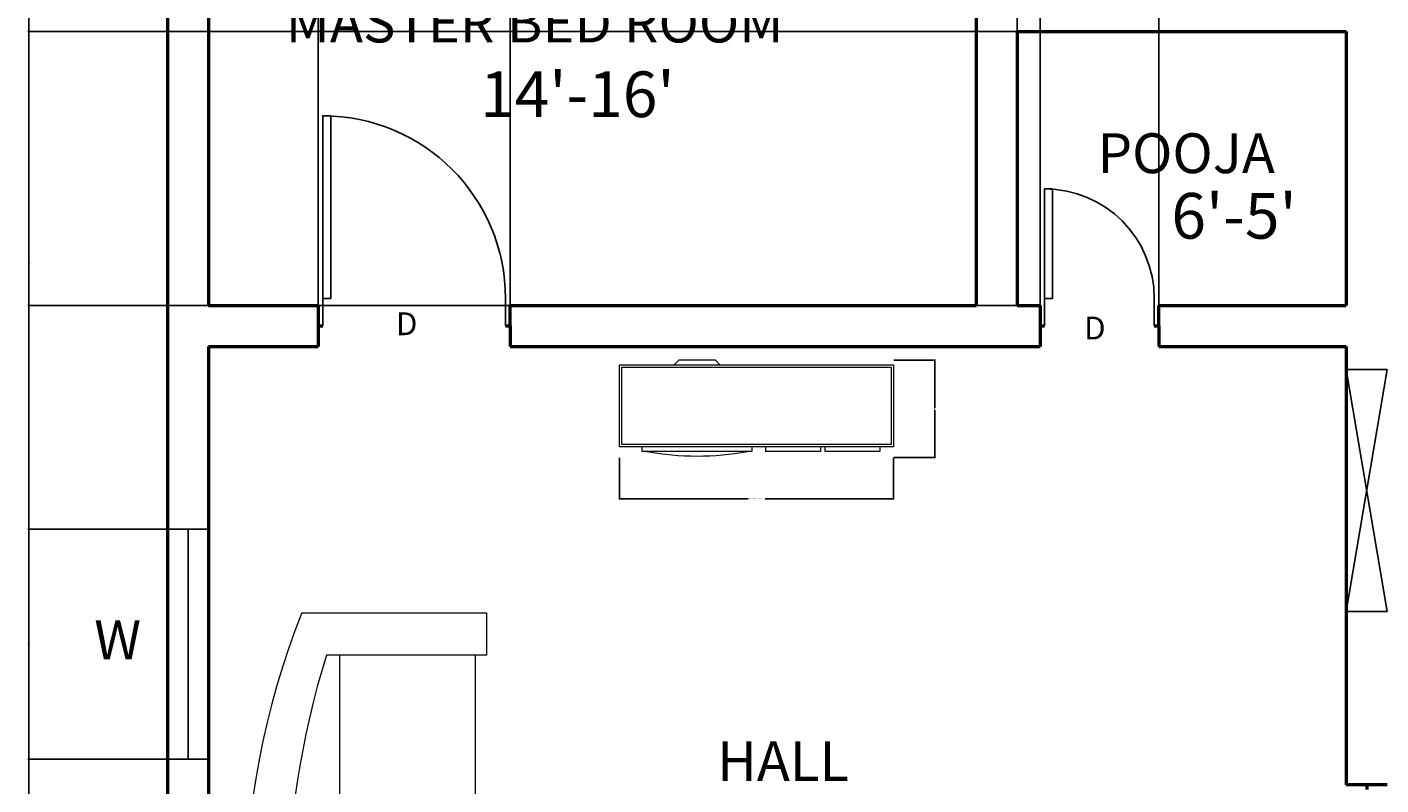
# Model space of a CAD drawing. Units: inches. Extents: x 2164 to 3752, y 2015 to 2629.
# Tile 2 of 8: x 2164 to 2461, y 2223 to 2389. Entities that reach past the tile are written whole.
import ezdxf
from ezdxf.enums import TextEntityAlignment as Align

# ---------------------------------------------------------------- set-up
doc = ezdxf.new("R2010")
doc.units = ezdxf.units.IN
for name, color, linetype, lineweight in [('A-ANNO-DIMS', 2, 'Continuous', 18), ('A-ANNO-TEXT', 7, 'Continuous', 25), ('A-AREA-IDEN', 3, 'Continuous', 25), ('A-DOOR', 3, 'Continuous', 25), ('A-FURN', 8, 'Continuous', 18), ('A-GLAZ', 4, 'Continuous', 25), ('A-WALL', 7, 'Continuous', 50)]:
    doc.layers.add(name, color=color, linetype=linetype, lineweight=lineweight)
doc.styles.get("Standard").update_dxf_attribs({"font": 'arial.ttf'})
doc.dimstyles.get("Standard").update_dxf_attribs({"dimtxt": 0.18, "dimasz": 0.18, "dimexe": 0.18, "dimexo": 0.0625, "dimgap": 0.09, "dimtad": 0, "dimtih": 1, "dimtoh": 1, "dimdec": 4, "dimzin": 0, "dimdsep": 46, "dimtxsty": 'Standard', "dimcen": 0.09, "dimadec": 0, "dimazin": 0, "dimtfac": 1, "dimtdec": 4, "dimtofl": 0, "dimtmove": 0, "dimatfit": 3, "dimfxl": 1, "dimtolj": 1, "dimtzin": 0, "dimarcsym": 0})

# ---------------------------------------------------------------- blocks, each defined once
blk = doc.blocks.new('Sofa - Roundback 7 ft.')
for p, q in [((-12.00002, -32.4421), (-12.00003, -6.5971)), ((11.99997, -32.4421), (11.99998, -6.5971)), ((-36.000027, -34), (-36.000027, -11.4696)), ((35.99998, -34), (35.99998, -11.4696)), ((-35.999844, -13.3819), (35.9998, -13.3819)), ((-36.000027, -32.4421), (35.99998, -32.4421))]:
    blk.add_line(p, q)
for points in [[(-36.000027, -34), (-42.000027, -34), (-42.000027, -8)], [(41.99998, -8), (41.99998, -34), (35.99998, -34)]]:
    blk.add_lwpolyline(points)
for centre, radius, start, end in [((0, -114.25), 114.25, 68.43141, 111.5686), ((-0.00001, -127.1968), 121.1968, 72.72033, 107.2797)]:
    blk.add_arc(centre, radius, start, end)
blk = doc.blocks.new('*U2')
for p, q in [((0, 0), (0, -6)), ((24, 0), (24, -6))]:
    blk.add_line(p, q)
blk.add_lwpolyline([(0, 0), (0, 24), (1.75, 24), (1.75, 0)], close=True)
blk.add_arc((0, 0), 24, 0, 90)
blk = doc.blocks.new('Entertainment Center')
for p, q in [((-4, 0), (-5, -1)), ((4, 0), (-4, 0)), ((5, -1), (4, 0)), ((-17, -19), (-17, -1)), ((-17, -1), (43, -1)), ((-16.5, -18.5), (-16.5, -1.5)), ((-16.5, -1.5), (42.5, -1.5)), ((42.5, -1.5), (42.5, -18.5)), ((43, -1), (43, -19)), ((43, -19), (-17, -19)), ((42.5, -18.5), (-16.5, -18.5)), ((-12, -20), (-12, -19)), ((12, -20), (-12, -20)), ((12, -19), (12, -20)), ((15, -20), (15, -19)), ((27, -20), (15, -20)), ((27, -19), (27, -20)), ((28, -20), (28, -19)), ((40, -20), (28, -20)), ((40, -19), (40, -20))]:
    blk.add_line(p, q)
blk.add_arc((0, 40), 61, 259.6111, 280.3889)
blk = doc.blocks.new('*U7')
for p, q in [((0, 0), (0, -6)), ((40, 0), (40, -6))]:
    blk.add_line(p, q)
blk.add_lwpolyline([(0, 0), (0, 40), (1.75, 40), (1.75, 0)], close=True)
blk.add_arc((0, 0), 40, 0, 90)
blk = doc.blocks.new('VENT-OPENING')
for p, q in [((9, 53), (0, 53)), ((9, 53), (0, 0)), ((9, 0), (0, 53)), ((9, 0), (0, 0))]:
    blk.add_line(p, q)
blk = doc.blocks.new('*D43')
at = {"layer": 'A-ANNO-DIMS', "color": 0, "lineweight": -2, "transparency": 16777216}
for p, q in [((2294.06, 2294.33), (2294.06, 2285.21)), ((2354.06, 2294.33), (2354.06, 2285.21)), ((2294.24, 2285.39), (2322.19, 2285.39)), ((2353.88, 2285.39), (2325.93, 2285.39))]:
    blk.add_line(p, q, dxfattribs=at)
at = {"layer": 'A-ANNO-DIMS', "color": 0, "transparency": 16777216}
for points in [[(2294.24, 2285.42), (2294.24, 2285.36), (2294.06, 2285.39)], [(2353.88, 2285.42), (2353.88, 2285.36), (2354.06, 2285.39)]]:
    blk.add_solid(points, dxfattribs=at)
at = {"layer": 'Defpoints', "color": 0, "transparency": 16777216}
for p in [(2294.06, 2294.39), (2354.06, 2294.39), (2354.06, 2285.39)]:
    blk.add_point(p, dxfattribs=at)
at = {"layer": 'A-ANNO-DIMS', "color": 0, "transparency": 16777216, "insert": (2324.06, 2285.39), "char_height": 0.18, "attachment_point": 5}
blk.add_mtext('\\A1;ENTERTAINMENT CENTER 60', dxfattribs=at)
blk = doc.blocks.new('*D44')
at = {"layer": 'A-ANNO-DIMS', "color": 0, "lineweight": -2, "transparency": 16777216}
for p, q in [((2354.12, 2315.73), (2363.24, 2315.73)), ((2363.06, 2315.55), (2363.06, 2305.24)), ((2363.06, 2294.57), (2363.06, 2304.88)), ((2354.12, 2294.39), (2363.24, 2294.39))]:
    blk.add_line(p, q, dxfattribs=at)
at = {"layer": 'A-ANNO-DIMS', "color": 0, "transparency": 16777216}
for points in [[(2363.03, 2315.55), (2363.09, 2315.55), (2363.06, 2315.73)], [(2363.03, 2294.57), (2363.09, 2294.57), (2363.06, 2294.39)]]:
    blk.add_solid(points, dxfattribs=at)
at = {"layer": 'Defpoints', "color": 0, "transparency": 16777216}
for p in [(2354.06, 2315.73), (2363.06, 2315.73), (2354.06, 2294.39)]:
    blk.add_point(p, dxfattribs=at)
at = {"layer": 'A-ANNO-DIMS', "color": 0, "transparency": 16777216, "insert": (2363.06, 2305.06), "char_height": 0.18, "attachment_point": 5}
blk.add_mtext('\\A1;21', dxfattribs=at)
blk = doc.blocks.new('*D70')
at = {"layer": 'A-ANNO-DIMS', "color": 0, "lineweight": -2, "transparency": 16777216}
for p, q in [((2195.05, 2228.35), (2164.58, 2228.35)), ((2164.76, 2228.17), (2164.76, 2202)), ((2164.76, 2175.46), (2164.76, 2201.63)), ((2195.05, 2175.28), (2164.58, 2175.28))]:
    blk.add_line(p, q, dxfattribs=at)
at = {"layer": 'A-ANNO-DIMS', "color": 0, "transparency": 16777216}
for points in [[(2164.73, 2228.17), (2164.79, 2228.17), (2164.76, 2228.35)], [(2164.73, 2175.46), (2164.79, 2175.46), (2164.76, 2175.28)]]:
    blk.add_solid(points, dxfattribs=at)
at = {"layer": 'Defpoints', "color": 0, "transparency": 16777216}
for p in [(2164.76, 2228.35), (2195.11, 2228.35), (2195.11, 2175.28)]:
    blk.add_point(p, dxfattribs=at)
at = {"layer": 'A-ANNO-DIMS', "color": 0, "transparency": 16777216, "insert": (2164.76, 2201.82), "char_height": 0.18, "attachment_point": 5}
blk.add_mtext('\\A1;53.07', dxfattribs=at)
blk = doc.blocks.new('*D71')
at = {"layer": 'A-ANNO-DIMS', "color": 0, "lineweight": -2, "transparency": 16777216}
for p, q in [((2195.05, 2278.69), (2164.58, 2278.69)), ((2164.76, 2278.51), (2164.76, 2253.7)), ((2164.76, 2228.53), (2164.76, 2253.34)), ((2195.05, 2228.35), (2164.58, 2228.35))]:
    blk.add_line(p, q, dxfattribs=at)
at = {"layer": 'A-ANNO-DIMS', "color": 0, "transparency": 16777216}
for points in [[(2164.73, 2278.51), (2164.79, 2278.51), (2164.76, 2278.69)], [(2164.73, 2228.53), (2164.79, 2228.53), (2164.76, 2228.35)]]:
    blk.add_solid(points, dxfattribs=at)
at = {"layer": 'Defpoints', "color": 0, "transparency": 16777216}
for p in [(2164.76, 2278.69), (2195.11, 2278.69), (2195.11, 2228.35)]:
    blk.add_point(p, dxfattribs=at)
at = {"layer": 'A-ANNO-DIMS', "color": 0, "transparency": 16777216, "insert": (2164.76, 2253.52), "char_height": 0.18, "attachment_point": 5}
blk.add_mtext('\\A1;50.34', dxfattribs=at)
blk = doc.blocks.new('*D72')
at = {"layer": 'A-ANNO-DIMS', "color": 0, "lineweight": -2, "transparency": 16777216}
for p, q in [((2195.05, 2395.15), (2164.58, 2395.15)), ((2164.76, 2394.97), (2164.76, 2337.1)), ((2164.76, 2278.87), (2164.76, 2336.74)), ((2195.05, 2278.69), (2164.58, 2278.69))]:
    blk.add_line(p, q, dxfattribs=at)
at = {"layer": 'A-ANNO-DIMS', "color": 0, "transparency": 16777216}
for points in [[(2164.73, 2394.97), (2164.79, 2394.97), (2164.76, 2395.15)], [(2164.73, 2278.87), (2164.79, 2278.87), (2164.76, 2278.69)]]:
    blk.add_solid(points, dxfattribs=at)
at = {"layer": 'Defpoints', "color": 0, "transparency": 16777216}
for p in [(2164.76, 2395.15), (2195.11, 2395.15), (2195.11, 2278.69)]:
    blk.add_point(p, dxfattribs=at)
at = {"layer": 'A-ANNO-DIMS', "color": 0, "transparency": 16777216, "insert": (2164.76, 2336.92), "char_height": 0.18, "attachment_point": 5}
blk.add_mtext('\\A1;116.47', dxfattribs=at)
blk = doc.blocks.new('*D75')
at = {"layer": 'A-ANNO-DIMS', "color": 0, "lineweight": -2, "transparency": 16777216}
for p, q in [((2195.05, 2528.72), (2164.58, 2528.72)), ((2164.76, 2528.54), (2164.76, 2287.4)), ((2164.76, 2045.9), (2164.76, 2287.04)), ((2195.05, 2045.72), (2164.58, 2045.72))]:
    blk.add_line(p, q, dxfattribs=at)
at = {"layer": 'A-ANNO-DIMS', "color": 0, "transparency": 16777216}
for points in [[(2164.73, 2528.54), (2164.79, 2528.54), (2164.76, 2528.72)], [(2164.73, 2045.9), (2164.79, 2045.9), (2164.76, 2045.72)]]:
    blk.add_solid(points, dxfattribs=at)
at = {"layer": 'Defpoints', "color": 0, "transparency": 16777216}
for p in [(2164.76, 2528.72), (2195.11, 2528.72), (2195.11, 2045.72)]:
    blk.add_point(p, dxfattribs=at)
at = {"layer": 'A-ANNO-DIMS', "color": 0, "transparency": 16777216, "insert": (2164.76, 2287.22), "char_height": 0.18, "attachment_point": 5}
blk.add_mtext('\\A1;483', dxfattribs=at)
blk = doc.blocks.new('*D87')
at = {"layer": 'A-ANNO-DIMS', "color": 0, "lineweight": -2, "transparency": 16777216}
for p, q in [((2381.05, 2387.72), (2164.58, 2387.72)), ((2164.76, 2387.54), (2164.76, 2357.9)), ((2164.76, 2327.9), (2164.76, 2357.54)), ((2381.05, 2327.72), (2164.58, 2327.72))]:
    blk.add_line(p, q, dxfattribs=at)
at = {"layer": 'A-ANNO-DIMS', "color": 0, "transparency": 16777216}
for points in [[(2164.73, 2387.54), (2164.79, 2387.54), (2164.76, 2387.72)], [(2164.73, 2327.9), (2164.79, 2327.9), (2164.76, 2327.72)]]:
    blk.add_solid(points, dxfattribs=at)
at = {"layer": 'Defpoints', "color": 0, "transparency": 16777216}
for p in [(2164.76, 2387.72), (2381.11, 2387.72), (2381.11, 2327.72)]:
    blk.add_point(p, dxfattribs=at)
at = {"layer": 'A-ANNO-DIMS', "color": 0, "transparency": 16777216, "insert": (2164.76, 2357.72), "char_height": 0.18, "attachment_point": 5}
blk.add_mtext('\\A1;60', dxfattribs=at)
blk = doc.blocks.new('*D88')
at = {"layer": 'A-ANNO-DIMS', "color": 0, "lineweight": -2, "transparency": 16777216}
for p, q in [((2381.05, 2393.72), (2164.58, 2393.72)), ((2164.76, 2393.54), (2164.76, 2390.9)), ((2164.76, 2387.9), (2164.76, 2390.54)), ((2381.05, 2387.72), (2164.58, 2387.72))]:
    blk.add_line(p, q, dxfattribs=at)
at = {"layer": 'A-ANNO-DIMS', "color": 0, "transparency": 16777216}
for points in [[(2164.73, 2393.54), (2164.79, 2393.54), (2164.76, 2393.72)], [(2164.73, 2387.9), (2164.79, 2387.9), (2164.76, 2387.72)]]:
    blk.add_solid(points, dxfattribs=at)
at = {"layer": 'Defpoints', "color": 0, "transparency": 16777216}
for p in [(2164.76, 2393.72), (2381.11, 2393.72), (2381.11, 2387.72)]:
    blk.add_point(p, dxfattribs=at)
at = {"layer": 'A-ANNO-DIMS', "color": 0, "transparency": 16777216, "insert": (2164.76, 2390.72), "char_height": 0.18, "attachment_point": 5}
blk.add_mtext('\\A1;6', dxfattribs=at)
blk = doc.blocks.new('*D92')
at = {"layer": 'A-ANNO-DIMS', "color": 0, "lineweight": -2, "transparency": 16777216}
for p, q in [((2228.11, 2327.78), (2228.11, 2559.25)), ((2228.29, 2559.07), (2248.89, 2559.07)), ((2269.93, 2559.07), (2249.33, 2559.07)), ((2270.11, 2327.78), (2270.11, 2559.25))]:
    blk.add_line(p, q, dxfattribs=at)
at = {"layer": 'A-ANNO-DIMS', "color": 0, "transparency": 16777216}
for points in [[(2228.29, 2559.1), (2228.29, 2559.04), (2228.11, 2559.07)], [(2269.93, 2559.1), (2269.93, 2559.04), (2270.11, 2559.07)]]:
    blk.add_solid(points, dxfattribs=at)
at = {"layer": 'Defpoints', "color": 0, "transparency": 16777216}
for p in [(2270.11, 2559.07), (2228.11, 2327.72), (2270.11, 2327.72)]:
    blk.add_point(p, dxfattribs=at)
at = {"layer": 'A-ANNO-DIMS', "color": 0, "transparency": 16777216, "insert": (2249.11, 2559.07), "char_height": 0.18, "attachment_point": 5}
blk.add_mtext('\\A1;42', dxfattribs=at)
blk = doc.blocks.new('*D93')
at = {"layer": 'A-ANNO-DIMS', "color": 0, "lineweight": -2, "transparency": 16777216}
for p, q in [((2381.11, 2327.78), (2381.11, 2559.25)), ((2381.29, 2559.07), (2383.46, 2559.07)), ((2385.93, 2559.07), (2383.76, 2559.07)), ((2386.11, 2327.78), (2386.11, 2559.25))]:
    blk.add_line(p, q, dxfattribs=at)
at = {"layer": 'A-ANNO-DIMS', "color": 0, "transparency": 16777216}
for points in [[(2381.29, 2559.1), (2381.29, 2559.04), (2381.11, 2559.07)], [(2385.93, 2559.1), (2385.93, 2559.04), (2386.11, 2559.07)]]:
    blk.add_solid(points, dxfattribs=at)
at = {"layer": 'Defpoints', "color": 0, "transparency": 16777216}
for p in [(2386.11, 2559.07), (2381.11, 2327.72), (2386.11, 2327.72)]:
    blk.add_point(p, dxfattribs=at)
at = {"layer": 'A-ANNO-DIMS', "color": 0, "transparency": 16777216, "insert": (2383.61, 2559.07), "char_height": 0.18, "attachment_point": 5}
blk.add_mtext('\\A1;5', dxfattribs=at)
blk = doc.blocks.new('*D94')
at = {"layer": 'A-ANNO-DIMS', "color": 0, "lineweight": -2, "transparency": 16777216}
for p, q in [((2386.11, 2327.78), (2386.11, 2559.25)), ((2386.29, 2559.07), (2398.89, 2559.07)), ((2411.93, 2559.07), (2399.33, 2559.07)), ((2412.11, 2327.78), (2412.11, 2559.25))]:
    blk.add_line(p, q, dxfattribs=at)
at = {"layer": 'A-ANNO-DIMS', "color": 0, "transparency": 16777216}
for points in [[(2386.29, 2559.1), (2386.29, 2559.04), (2386.11, 2559.07)], [(2411.93, 2559.1), (2411.93, 2559.04), (2412.11, 2559.07)]]:
    blk.add_solid(points, dxfattribs=at)
at = {"layer": 'Defpoints', "color": 0, "transparency": 16777216}
for p in [(2412.11, 2559.07), (2386.11, 2327.72), (2412.11, 2327.72)]:
    blk.add_point(p, dxfattribs=at)
at = {"layer": 'A-ANNO-DIMS', "color": 0, "transparency": 16777216, "insert": (2399.11, 2559.07), "char_height": 0.18, "attachment_point": 5}
blk.add_mtext('\\A1;26', dxfattribs=at)

msp = doc.modelspace()

# ---------------------------------------------------------------- linework, layer by layer
at = {"layer": 'A-GLAZ'}
for p, q in [((2195.1113, 2278.6856), (2204.1113, 2278.6856)), ((2199.6113, 2228.3505), (2199.6113, 2278.6856)), ((2195.1113, 2228.3505), (2204.1113, 2228.3505))]:
    msp.add_line(p, q, dxfattribs=at)
at = {"layer": 'A-WALL'}
for p, q in [((2195.1113, 2528.7172), (2195.1113, 2045.7172)), ((2204.1113, 2519.7172), (2204.1113, 2327.7172)), ((2372.1113, 2464.7172), (2372.1113, 2327.7172)), ((2381.1113, 2387.7172), (2453.1113, 2387.7172)), ((2381.1113, 2387.7172), (2381.1113, 2370.7172)), ((2381.1113, 2387.7172), (2381.1113, 2327.7172)), ((2453.1113, 2387.7172), (2453.1113, 2327.7172)), ((2372.1113, 2332.7172), (2372.1113, 2327.7172)), ((2453.1113, 2332.7172), (2453.1113, 2327.7172)), ((2204.1113, 2327.7172), (2228.1113, 2327.7172)), ((2228.1113, 2327.7172), (2228.1113, 2318.7172)), ((2270.1108, 2323.2593), (2270.1108, 2327.7172)), ((2270.1108, 2327.7172), (2372.1113, 2327.7172)), ((2381.1113, 2327.7172), (2386.1113, 2327.7172)), ((2386.1113, 2327.7172), (2386.1113, 2318.7172)), ((2412.1111, 2323.2346), (2412.1111, 2327.7172)), ((2412.1111, 2327.7172), (2453.1113, 2327.7172)), ((2228.1113, 2323.2172), (2229.1112, 2323.2337)), ((2269.1112, 2323.2337), (2270.1108, 2323.2593)), ((2270.1108, 2323.2593), (2270.1108, 2318.7172)), ((2386.1113, 2323.2172), (2387.1111, 2323.2346)), ((2411.1111, 2323.2346), (2412.1111, 2323.2346)), ((2412.1111, 2323.2346), (2412.1111, 2318.7172)), ((2204.1113, 2318.7172), (2228.1113, 2318.7172)), ((2204.1113, 2318.7172), (2204.1113, 2054.7172)), ((2270.1108, 2318.7172), (2386.1113, 2318.7172)), ((2381.1113, 2318.7172), (2386.1113, 2318.7172)), ((2412.1111, 2318.7172), (2453.1113, 2318.7172)), ((2412.1111, 2318.7172), (2453.1113, 2318.7172)), ((2453.1113, 2318.7172), (2453.1113, 2222.7172)), ((2462.1113, 2222.7172), (2453.1113, 2222.7172)), ((2457.6113, 2222.7172), (2457.6113, 2221.7172))]:
    msp.add_line(p, q, dxfattribs=at)

# ---------------------------------------------------------------- block references
at = {"layer": 'A-DOOR'}
for name, p in [('*U7', (2229.1112, 2329.2337)), ('*U2', (2387.1111, 2329.2346))]:
    msp.add_blockref(name, p, dxfattribs=at)
at = {"layer": 'A-FURN'}
msp.add_blockref('Entertainment Center', (2311.0587, 2315.7266), dxfattribs=at)
at = {"layer": 'A-FURN', "xscale": 1.554837866346122, "yscale": 1.554837866346122, "zscale": 1.554837866346122, "rotation": 90}
msp.add_blockref('Sofa - Roundback 7 ft.', (2212.0723, 2195.1336), dxfattribs=at)
at = {"layer": 'A-GLAZ'}
msp.add_blockref('VENT-OPENING', (2453.1113, 2260.717), dxfattribs=at)

# ---------------------------------------------------------------- texts
at = {"layer": 'A-ANNO-TEXT'}
for p in [(2245.1325, 2321.1958), (2395.7692, 2320.251)]:
    msp.add_text('D', height=5, dxfattribs=at).set_placement(p)
msp.add_text('W', height=8.5558, dxfattribs=at).set_placement((2184.2104, 2253.3664), align=Align.MIDDLE)
at = {"layer": 'A-AREA-IDEN'}
for s, height, p in [('MASTER BED ROOM', 8.722848, (2221.017, 2385.2901)), ("14'-16'", 10, (2263.5413, 2368.9464)), ('POOJA', 8.72285, (2398.7289, 2356.6782)), ("6'-5'", 10, (2414.8622, 2342.3341)), ('HALL', 8.72285, (2315.4619, 2223.5733))]:
    msp.add_text(s, height=height, dxfattribs=at).set_placement(p)

# ---------------------------------------------------------------- dimensions: what is measured, and where the dimension line sits
at = {"layer": 'A-ANNO-DIMS'}
for base, p1, p2, picture, middle in [((2270.1108, 2559.0672), (2228.1113, 2327.7172), (2270.1108, 2327.7172), '*D92', (2249.1111, 2559.0672)), ((2386.1113, 2559.0672), (2381.1113, 2327.7172), (2386.1113, 2327.7172), '*D93', (2383.6113, 2559.0672)), ((2412.1111, 2559.0672), (2386.1113, 2327.7172), (2412.1111, 2327.7172), '*D94', (2399.1112, 2559.0672))]:
    dim = msp.add_linear_dim(base=base, p1=p1, p2=p2, dimstyle='Standard', override={"dimdec": 0, "dimlfac": 1, "dimrnd": 0, "dimzin": 0, "dimdsep": 46, "dimlunit": 2}, dxfattribs=at)
    dim.commit()
    dim.dimension.update_dxf_attribs({"geometry": picture, "text_midpoint": middle})
for base, p1, p2, override, picture, middle in [((2164.7613, 2528.7172), (2195.1113, 2045.7172), (2195.1113, 2528.7172), {"dimdec": 0, "dimlfac": 1, "dimrnd": 0, "dimzin": 0, "dimdsep": 46, "dimlunit": 2}, '*D75', (2164.7613, 2287.2172)), ((2164.7613, 2395.1516), (2195.1113, 2278.6856), (2195.1113, 2395.1516), {"dimdec": 2, "dimlfac": 1, "dimrnd": 0, "dimzin": 0, "dimdsep": 46, "dimlunit": 2}, '*D72', (2164.7613, 2336.9186)), ((2164.7613, 2393.7172), (2381.1113, 2387.7172), (2381.1113, 2393.7172), {"dimdec": 0, "dimlfac": 1, "dimrnd": 0, "dimzin": 0, "dimdsep": 46, "dimlunit": 2}, '*D88', (2164.7613, 2390.7172)), ((2164.7613, 2387.7172), (2381.1113, 2327.7172), (2381.1113, 2387.7172), {"dimdec": 0, "dimlfac": 1, "dimrnd": 0, "dimzin": 0, "dimdsep": 46, "dimlunit": 2}, '*D87', (2164.7613, 2357.7172)), ((2363.0587, 2315.7266), (2354.0587, 2294.3933), (2354.0587, 2315.7266), {"dimdec": 0, "dimrnd": 0, "dimzin": 0, "dimlunit": 2}, '*D44', (2363.0587, 2305.0599)), ((2164.7613, 2278.6856), (2195.1113, 2228.3505), (2195.1113, 2278.6856), {"dimdec": 2, "dimlfac": 1, "dimrnd": 0, "dimzin": 0, "dimdsep": 46, "dimlunit": 2}, '*D71', (2164.7613, 2253.5181)), ((2164.7613, 2228.3505), (2195.1113, 2175.28), (2195.1113, 2228.3505), {"dimdec": 2, "dimlfac": 1, "dimrnd": 0, "dimzin": 0, "dimdsep": 46, "dimlunit": 2}, '*D70', (2164.7613, 2201.8152))]:
    dim = msp.add_linear_dim(base=base, p1=p1, p2=p2, angle=90, dimstyle='Standard', override=override, dxfattribs=at)
    dim.commit()
    dim.dimension.update_dxf_attribs({"geometry": picture, "text_midpoint": middle})
dim = msp.add_linear_dim(base=(2354.0587, 2285.3933), p1=(2294.0587, 2294.3933), p2=(2354.0587, 2294.3933), text='ENTERTAINMENT CENTER <>', dimstyle='Standard', override={"dimdec": 0, "dimrnd": 0, "dimzin": 0, "dimlunit": 2}, dxfattribs=at)
dim.commit()
dim.dimension.update_dxf_attribs({"geometry": '*D43', "text_midpoint": (2324.0587, 2285.3933)})

doc.saveas('drawing.dxf')
